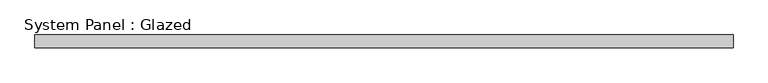
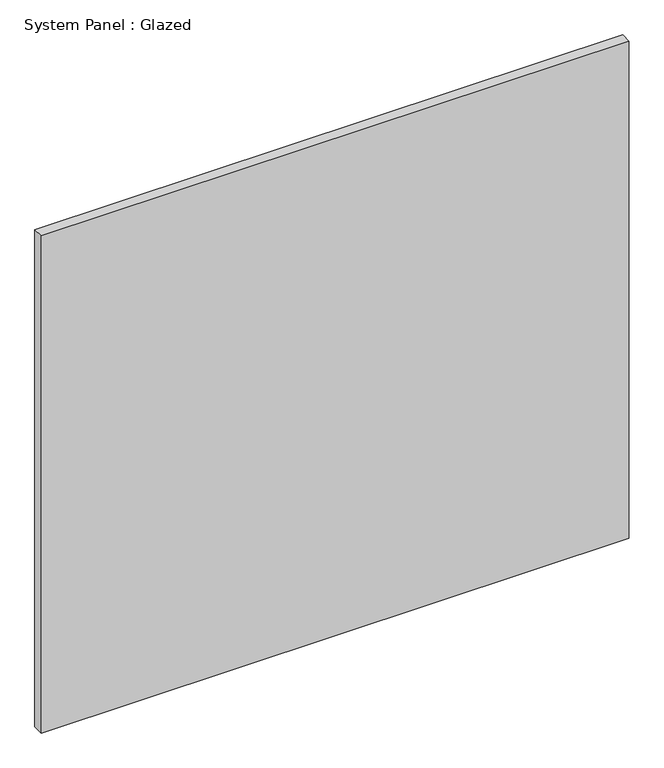
"""IFC4 building model written with IfcOpenShell, lengths in millimetres: plate geometry, System Panel : Glazed."""

from ifc_helpers import new_model, si_unit, origin, origin_with_axes, place, context, project, spatial, polyline, outline, extrude, source, transform, mapped, element, save


def system_panel_glazed_67cddadf(model_context):
    return source(origin(), model_context, "Body", "SweptSolid", [
        extrude(outline(polyline([(682.1772472, 19.05), (-682.1772472, 19.05), (-682.1772472, 44.45), (682.1772472, 44.45), (682.1772472, 19.05)])), origin_with_axes(), (0.0, 0.0, 1.0), 1219.2),
    ])


if __name__ == "__main__":
    model = new_model("IFC4")
    model_context = context("Model", 3, world=origin())
    ifc_project = project(units=[si_unit("LENGTHUNIT", "METRE", prefix="MILLI")], contexts=[model_context])
    site = spatial("IfcSite", under=ifc_project)
    building = spatial("IfcBuilding", under=site)
    placement = place(None, origin())
    system_panel_glazed_shape = system_panel_glazed_67cddadf(model_context)
    element("IfcPlate", 1, ObjectType="System Panel : Glazed", at=placement, inside=building, context=model_context, shape_type="MappedRepresentation", body=[
        mapped(system_panel_glazed_shape, transform((0.0, 0.0, 0.0), x_axis=(1.0, 0.0, 0.0), y_axis=(0.0, 1.0, 0.0), z_axis=(0.0, 0.0, 1.0))),
    ])
    save(model, "model.ifc")

# Revit data of these elements
# Type "System Panel : Glazed"
#   Construction Type Id = "GSP4R"
#   Analytic Construction = "1/8 in Pilkington single glazing"
#   Visual Light Transmittance = 0.9
#   Solar Heat Gain Coefficient = 0.86
#   Heat Transfer Coefficient (U) = 1.18115 BTU/(h·ft²·°F)
# Element 1 (IfcPlate, "System Panel : Glazed")
#   Materials on its faces: "Glass"
# Materials
#   "Glass": class "Glass", colour RGB 0 128 192, transparency 0.75, Description = "Soda Lime Glass", Cost = 0
